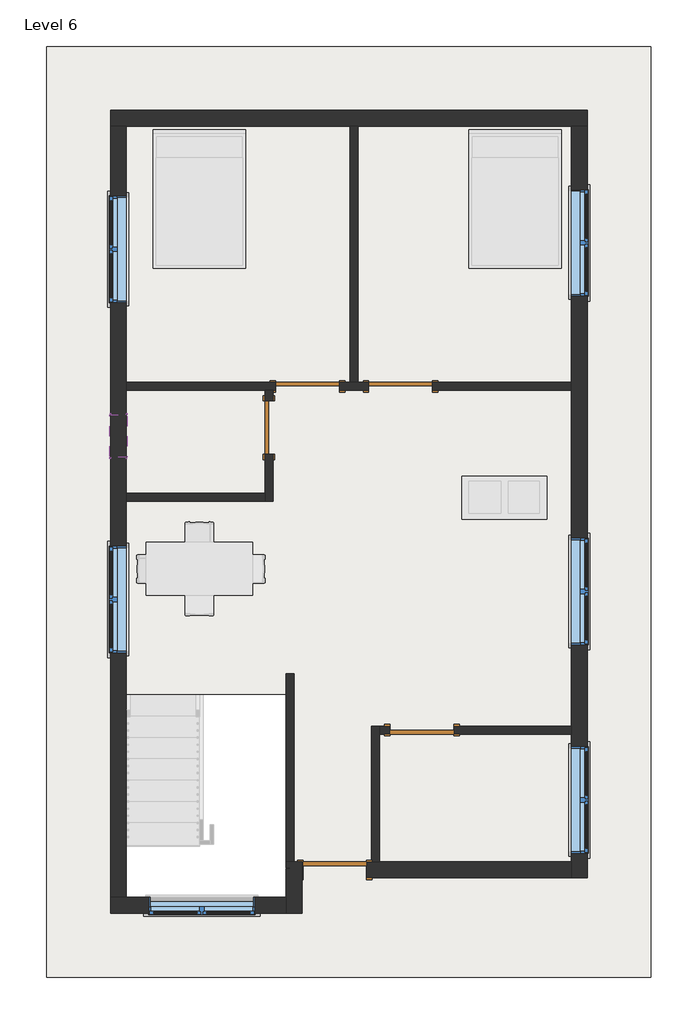
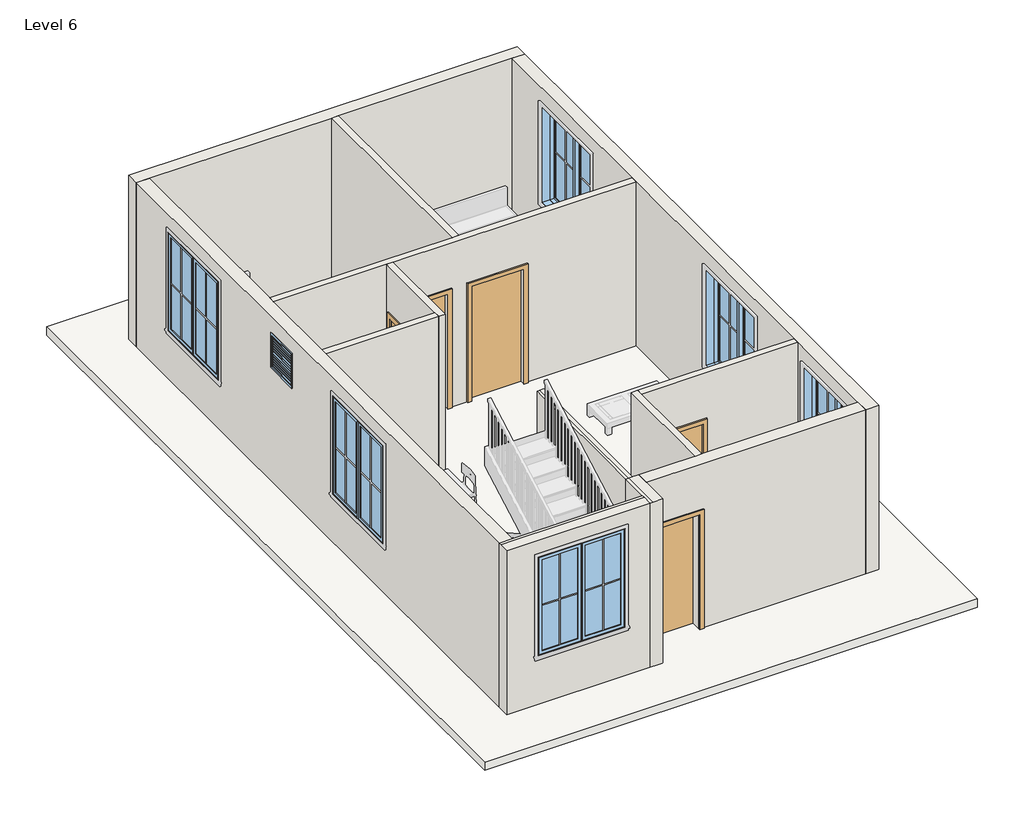
# One storey, part 1 of 3: 13 walls, 7 windows, 5 doors, 1 roof.
"""IFC4 building model written with IfcOpenShell, lengths in millimetres."""

from ifc_helpers import new_model, si_unit, frame, origin, place, context, project, spatial, polyline, outline, extrude, faceted_brep, transform, mapped, element, save
from components import door_214872d5, single_flush_door_3_e5f9f3c4, single_flush_door_3_305aa2a5, single_flush_door_3_0ca8825f, window_casement_double_win_5_f93960c7, window_f2d8fef0

model = new_model("IFC4")

# Units and contexts
model_context = context("Model", 3, world=origin())
ifc_project = project(units=[si_unit("LENGTHUNIT", "METRE", prefix="MILLI")], contexts=[model_context])

# Site, building, storey
site = spatial("IfcSite", under=ifc_project)
building = spatial("IfcBuilding", under=site)
storey = spatial("IfcBuildingStorey", under=building, Name="Level 6", Elevation=15849.6)

# Doors
placement = place(None, origin())
door_shape = door_214872d5(model_context)
element("IfcDoor", 1, ObjectType="Single-Flush : DOOR 2'6\"", at=placement, inside=storey, context=model_context, shape_type="MappedRepresentation", body=[
    mapped(door_shape, transform((-2193.930864, 251.0919982, 15849.6), x_axis=(0.0, 1.0, 0.0), y_axis=(-1.0, 0.0, 0.0), z_axis=(0.0, 0.0, 1.0))),
])
single_flush_door_3_shape = single_flush_door_3_e5f9f3c4(model_context)
element("IfcDoor", 2, ObjectType="Single-Flush : DOOR 3'", at=placement, inside=storey, context=model_context, shape_type="MappedRepresentation", body=[
    mapped(single_flush_door_3_shape, transform((-1641.3962678, 841.6419982, 15849.6), x_axis=(1.0, 0.0, 0.0), y_axis=(0.0, 1.0, 0.0), z_axis=(0.0, 0.0, 1.0))),
])
element("IfcDoor", 3, ObjectType="Single-Flush : DOOR 3'", at=placement, inside=storey, context=model_context, shape_type="MappedRepresentation", body=[
    mapped(single_flush_door_3_shape, transform((-3.180864, -4073.2580018, 15849.6), x_axis=(-1.0, 0.0, 0.0), y_axis=(0.0, -1.0, 0.0), z_axis=(0.0, 0.0, 1.0))),
])
single_flush_door_3_2_shape = single_flush_door_3_305aa2a5(model_context)
element("IfcDoor", 4, ObjectType="Single-Flush : DOOR 3'", at=placement, inside=storey, context=model_context, shape_type="MappedRepresentation", body=[
    mapped(single_flush_door_3_2_shape, transform((-307.980864, 841.6419982, 15849.6), x_axis=(-1.0, 0.0, 0.0), y_axis=(0.0, -1.0, 0.0), z_axis=(0.0, 0.0, 1.0))),
])
single_flush_door_3_3_shape = single_flush_door_3_0ca8825f(model_context)
element("IfcDoor", 5, ObjectType="Single-Flush : DOOR 3'", at=placement, inside=storey, context=model_context, shape_type="MappedRepresentation", body=[
    mapped(single_flush_door_3_3_shape, transform((-1250.955864, -6073.5080018, 15849.6), x_axis=(1.0, 0.0, 0.0), y_axis=(0.0, 1.0, 0.0), z_axis=(0.0, 0.0, 1.0))),
])

# Roof
element("IfcRoof", 6, ObjectType="ROOF 6\"", at=placement, inside=storey, context=model_context, shape_type="SweptSolid", body=[
    extrude(outline(polyline([(3273.419136, 5699.3919982), (3273.419136, -7610.2080018), (-5375.280864, -7610.2080018), (-5375.280864, 5699.3919982), (3273.419136, 5699.3919982)]), holes=[polyline([(-1895.480864, -3571.6080018), (-4232.280864, -3571.6080018), (-4232.280864, -6518.0080018), (-1895.480864, -6518.0080018), (-1895.480864, -3571.6080018)])]), frame((0.0, 0.0, 15697.2), z_axis=(0.0, 0.0, 1.0), x_axis=(1.0, 0.0, 0.0)), (0.0, 0.0, 1.0), 152.4),
])

# Walls
element("IfcWall", 7, ObjectType="WALL 4.5\"", at=placement, inside=storey, context=model_context, shape_type="SweptSolid", body=[
    extrude(outline(polyline([(-1031.880864, 898.7919982), (-1031.880864, 4556.3919982), (-917.580864, 4556.3919982), (-917.580864, 898.7919982), (-1031.880864, 898.7919982)])), frame((0.0, 0.0, 15849.6), z_axis=(0.0, 0.0, 1.0), x_axis=(1.0, 0.0, 0.0)), (0.0, 0.0, 1.0), 3048.0),
])
element("IfcWall", 8, ObjectType="WALL 4.5\"", at=placement, inside=storey, context=model_context, shape_type="Brep", body=[
    faceted_brep([(-765.180864, 898.7919982, 17983.2), (-765.180864, 898.7919982, 15849.6), (-917.580864, 898.7919982, 15849.6), (-1031.880864, 898.7919982, 15849.6), (-1184.1962678, 898.7919982, 15849.6), (-1184.1962678, 898.7919982, 17983.2), (-2098.5962678, 898.7919982, 17983.2), (-2098.5962678, 898.7919982, 15849.6), (-4232.280864, 898.7919982, 15849.6), (-4232.280864, 898.7919982, 18897.6), (-1031.880864, 898.7919982, 18897.6), (-917.580864, 898.7919982, 18897.6), (2130.419136, 898.7919982, 18897.6), (2130.419136, 898.7919982, 15849.6), (149.219136, 898.7919982, 15849.6), (149.219136, 898.7919982, 17983.2), (-1184.1962678, 784.4919982, 15849.6), (-765.180864, 784.4919982, 15849.6), (-765.180864, 784.4919982, 17983.2), (149.219136, 784.4919982, 17983.2), (149.219136, 784.4919982, 15849.6), (2130.419136, 784.4919982, 15849.6), (2130.419136, 784.4919982, 18897.6), (-2136.780864, 784.4919982, 18897.6), (-2251.080864, 784.4919982, 18897.6), (-4232.280864, 784.4919982, 18897.6), (-4232.280864, 784.4919982, 15849.6), (-2251.080864, 784.4919982, 15849.6), (-2136.780864, 784.4919982, 15849.6), (-2098.5962678, 784.4919982, 15849.6), (-2098.5962678, 784.4919982, 17983.2), (-1184.1962678, 784.4919982, 17983.2)], [[[0, 1, 2, 3, 4, 5, 6, 7, 8, 9, 10, 11, 12, 13, 14, 15]], [[16, 17, 18, 19, 20, 21, 22, 23, 24, 25, 26, 27, 28, 29, 30, 31]], [[29, 28, 27, 26, 8, 7]], [[14, 13, 21, 20]], [[4, 3, 2, 1, 17, 16]], [[13, 12, 22, 21]], [[9, 8, 26, 25]], [[5, 4, 16, 31]], [[6, 5, 31, 30]], [[7, 6, 30, 29]], [[18, 17, 1, 0]], [[19, 18, 0, 15]], [[20, 19, 15, 14]], [[12, 11, 10, 9, 25, 24, 23, 22]]]),
])
element("IfcWall", 9, ObjectType="WALL 4.5\"", at=placement, inside=storey, context=model_context, shape_type="Brep", body=[
    faceted_brep([(-2251.080864, 784.4919982, 15849.6), (-2251.080864, 632.0919982, 15849.6), (-2251.080864, 632.0919982, 17983.2), (-2251.080864, -129.9080018, 17983.2), (-2251.080864, -129.9080018, 15849.6), (-2251.080864, -688.7080018, 15849.6), (-2251.080864, -803.0080018, 15849.6), (-2251.080864, -803.0080018, 18897.6), (-2251.080864, -688.7080018, 18897.6), (-2251.080864, 784.4919982, 18897.6), (-2136.780864, 632.0919982, 17983.2), (-2136.780864, 632.0919982, 15849.6), (-2136.780864, 784.4919982, 15849.6), (-2136.780864, 784.4919982, 18897.6), (-2136.780864, -803.0080018, 18897.6), (-2136.780864, -803.0080018, 15849.6), (-2136.780864, -129.9080018, 15849.6), (-2136.780864, -129.9080018, 17983.2)], [[[0, 1, 2, 3, 4, 5, 6, 7, 8, 9]], [[10, 11, 12, 13, 14, 15, 16, 17]], [[16, 15, 6, 5, 4]], [[12, 11, 1, 0]], [[0, 9, 13, 12]], [[7, 6, 15, 14]], [[2, 1, 11, 10]], [[3, 2, 10, 17]], [[4, 3, 17, 16]], [[9, 8, 7, 14, 13]]]),
])
element("IfcWall", 10, ObjectType="WALL 4.5\"", at=placement, inside=storey, context=model_context, shape_type="SweptSolid", body=[
    extrude(outline(polyline([(-4232.280864, -688.7080018), (-2251.080864, -688.7080018), (-2251.080864, -803.0080018), (-4232.280864, -803.0080018), (-4232.280864, -688.7080018)])), frame((0.0, 0.0, 15849.6), z_axis=(0.0, 0.0, 1.0), x_axis=(1.0, 0.0, 0.0)), (0.0, 0.0, 1.0), 3048.0),
])
element("IfcWall", 11, ObjectType="WALL 4.5\"", at=placement, inside=storey, context=model_context, shape_type="Brep", body=[
    faceted_brep([(-1831.980864, -5959.2080018, 15849.6), (-1831.980864, -3266.8080018, 15849.6), (-1831.980864, -3266.8080018, 18897.6), (-1831.980864, -5959.2080018, 18897.6), (-1946.280864, -5959.2080018, 15849.6), (-1946.280864, -5959.2080018, 18897.6), (-1946.280864, -3266.8080018, 18897.6), (-1946.280864, -3266.8080018, 15849.6), (-1895.480864, -3266.8080018, 18897.6), (-1895.480864, -5959.2080018, 18897.6), (-1895.480864, -3571.6080018, 18897.6)], [[[0, 1, 2, 3]], [[4, 5, 6, 7]], [[1, 0, 4, 7]], [[2, 1, 7, 6, 8]], [[0, 3, 9, 5, 4]], [[3, 2, 8, 10, 9]], [[8, 6, 5, 9, 10]]]),
])
element("IfcWall", 12, ObjectType="WALL 4.5\"", at=placement, inside=storey, context=model_context, shape_type="Brep", body=[
    faceted_brep([(-612.780864, -5959.2080018, 15849.6), (-612.780864, -4130.4080018, 15849.6), (-612.780864, -4016.1080018, 15849.6), (-612.780864, -4016.1080018, 18897.6), (-612.780864, -4130.4080018, 18897.6), (-612.780864, -5959.2080018, 18897.6), (-727.080864, -5959.2080018, 15849.6), (-727.080864, -5959.2080018, 18897.6), (-727.080864, -4016.1080018, 18897.6), (-727.080864, -4016.1080018, 15849.6)], [[[0, 1, 2, 3, 4, 5]], [[6, 7, 8, 9]], [[2, 1, 0, 6, 9]], [[0, 5, 7, 6]], [[3, 2, 9, 8]], [[5, 4, 3, 8, 7]]]),
])
element("IfcWall", 13, ObjectType="WALL 4.5\"", at=placement, inside=storey, context=model_context, shape_type="SweptSolid", body=[
    extrude(outline(polyline([(15849.6, -612.780864), (15849.6, -460.380864), (17983.2, -460.380864), (17983.2, 454.019136), (15849.6, 454.019136), (15849.6, 2130.419136), (18897.6, 2130.419136), (18897.6, -612.780864), (15849.6, -612.780864)])), frame((0.0, -4130.4080018, 0.0), z_axis=(0.0, 1.0, 0.0), x_axis=(0.0, 0.0, 1.0)), (0.0, 0.0, 1.0), 114.3),
])
element("IfcWall", 14, ObjectType="WALL 9\"", at=placement, inside=storey, context=model_context, shape_type="Brep", body=[
    faceted_brep([(-4460.880864, 4556.3919982, 15849.6), (-4232.280864, 4556.3919982, 15849.6), (-1031.880864, 4556.3919982, 15849.6), (-917.580864, 4556.3919982, 15849.6), (2130.419136, 4556.3919982, 15849.6), (2359.019136, 4556.3919982, 15849.6), (2359.019136, 4556.3919982, 18897.6), (2130.419136, 4556.3919982, 18897.6), (-917.580864, 4556.3919982, 18897.6), (-1031.880864, 4556.3919982, 18897.6), (-4232.280864, 4556.3919982, 18897.6), (-4460.880864, 4556.3919982, 18897.6), (-4460.880864, 4784.9919982, 15849.6), (-4460.880864, 4784.9919982, 18897.6), (2359.019136, 4784.9919982, 18897.6), (2359.019136, 4784.9919982, 15849.6)], [[[0, 1, 2, 3, 4, 5, 6, 7, 8, 9, 10, 11]], [[12, 13, 14, 15]], [[5, 4, 3, 2, 1, 0, 12, 15]], [[6, 5, 15, 14]], [[0, 11, 13, 12]], [[11, 10, 9, 8, 7, 6, 14, 13]]]),
])
element("IfcWall", 15, ObjectType="WALL 9\"", at=placement, inside=storey, context=model_context, shape_type="Brep", body=[
    faceted_brep([(2130.419136, 4556.3919982, 15849.6), (2130.419136, 898.7919982, 15849.6), (2130.419136, 784.4919982, 15849.6), (2130.419136, -4016.1080018, 15849.6), (2130.419136, -4130.4080018, 15849.6), (2130.419136, -5959.2080018, 15849.6), (2130.419136, -6187.8080018, 15849.6), (2130.419136, -6187.8080018, 18897.6), (2130.419136, -5959.2080018, 18897.6), (2130.419136, -4130.4080018, 18897.6), (2130.419136, -4016.1080018, 18897.6), (2130.419136, 784.4919982, 18897.6), (2130.419136, 898.7919982, 18897.6), (2130.419136, 4556.3919982, 18897.6), (2130.419136, -5835.3830018, 18592.8), (2130.419136, -5835.3830018, 16764.0), (2130.419136, -4311.3830018, 16764.0), (2130.419136, -4311.3830018, 18592.8), (2130.419136, -2854.0580018, 18592.8), (2130.419136, -2854.0580018, 16764.0), (2130.419136, -1330.0580018, 16764.0), (2130.419136, -1330.0580018, 18592.8), (2130.419136, 2130.6919982, 18592.8), (2130.419136, 2130.6919982, 16764.0), (2130.419136, 3654.6919982, 16764.0), (2130.419136, 3654.6919982, 18592.8), (2359.019136, 4556.3919982, 15849.6), (2359.019136, 4556.3919982, 18897.6), (2359.019136, -6187.8080018, 18897.6), (2359.019136, -6187.8080018, 15849.6), (2359.019136, -5835.3830018, 18592.8), (2359.019136, -4311.3830018, 18592.8), (2359.019136, -4311.3830018, 16764.0), (2359.019136, -5835.3830018, 16764.0), (2359.019136, -2854.0580018, 18592.8), (2359.019136, -1330.0580018, 18592.8), (2359.019136, -1330.0580018, 16764.0), (2359.019136, -2854.0580018, 16764.0), (2359.019136, 2130.6919982, 18592.8), (2359.019136, 3654.6919982, 18592.8), (2359.019136, 3654.6919982, 16764.0), (2359.019136, 2130.6919982, 16764.0)], [[[0, 1, 2, 3, 4, 5, 6, 7, 8, 9, 10, 11, 12, 13], [14, 15, 16, 17], [18, 19, 20, 21], [22, 23, 24, 25]], [[26, 27, 28, 29], [30, 31, 32, 33], [34, 35, 36, 37], [38, 39, 40, 41]], [[6, 5, 4, 3, 2, 1, 0, 26, 29]], [[0, 13, 27, 26]], [[7, 6, 29, 28]], [[15, 14, 30, 33]], [[16, 15, 33, 32]], [[17, 16, 32, 31]], [[14, 17, 31, 30]], [[19, 18, 34, 37]], [[20, 19, 37, 36]], [[21, 20, 36, 35]], [[18, 21, 35, 34]], [[23, 22, 38, 41]], [[24, 23, 41, 40]], [[25, 24, 40, 39]], [[22, 25, 39, 38]], [[13, 12, 11, 10, 9, 8, 7, 28, 27]]]),
])
element("IfcWall", 16, ObjectType="WALL 9\"", at=placement, inside=storey, context=model_context, shape_type="Brep", body=[
    faceted_brep([(2130.419136, -5959.2080018, 15849.6), (-612.780864, -5959.2080018, 15849.6), (-727.080864, -5959.2080018, 15849.6), (-793.755864, -5959.2080018, 15849.6), (-793.755864, -5959.2080018, 17983.2), (-1708.155864, -5959.2080018, 17983.2), (-1708.155864, -5959.2080018, 15849.6), (-1717.680864, -5959.2080018, 15849.6), (-1717.680864, -5959.2080018, 18897.6), (-727.080864, -5959.2080018, 18897.6), (-612.780864, -5959.2080018, 18897.6), (2130.419136, -5959.2080018, 18897.6), (-793.755864, -6187.8080018, 17983.2), (-793.755864, -6187.8080018, 15849.6), (2130.419136, -6187.8080018, 15849.6), (2130.419136, -6187.8080018, 18897.6), (-1717.680864, -6187.8080018, 18897.6), (-1717.680864, -6187.8080018, 15849.6), (-1708.155864, -6187.8080018, 15849.6), (-1708.155864, -6187.8080018, 17983.2)], [[[0, 1, 2, 3, 4, 5, 6, 7, 8, 9, 10, 11]], [[12, 13, 14, 15, 16, 17, 18, 19]], [[18, 17, 7, 6]], [[14, 13, 3, 2, 1, 0]], [[0, 11, 15, 14]], [[8, 7, 17, 16]], [[4, 3, 13, 12]], [[5, 4, 12, 19]], [[6, 5, 19, 18]], [[11, 10, 9, 8, 16, 15]]]),
])
element("IfcWall", 17, ObjectType="WALL 9\"", at=placement, inside=storey, context=model_context, shape_type="Brep", body=[
    faceted_brep([(-1946.280864, -5959.2080018, 15849.6), (-1946.280864, -6467.2080018, 15849.6), (-1946.280864, -6695.8080018, 15849.6), (-1946.280864, -6695.8080018, 18897.6), (-1946.280864, -6467.2080018, 18897.6), (-1946.280864, -5959.2080018, 18897.6), (-1717.680864, -5959.2080018, 15849.6), (-1717.680864, -5959.2080018, 18897.6), (-1717.680864, -6187.8080018, 18897.6), (-1717.680864, -6695.8080018, 18897.6), (-1717.680864, -6695.8080018, 15849.6), (-1717.680864, -6187.8080018, 15849.6), (-1831.980864, -5959.2080018, 15849.6), (-1895.480864, -5959.2080018, 18897.6), (-1831.980864, -5959.2080018, 18897.6), (-1895.480864, -6695.8080018, 18897.6), (-1895.480864, -6518.0080018, 18897.6)], [[[0, 1, 2, 3, 4, 5]], [[6, 7, 8, 9, 10, 11]], [[2, 1, 0, 12, 6, 11, 10]], [[0, 5, 13, 14, 7, 6, 12]], [[3, 2, 10, 9, 15]], [[5, 4, 3, 15, 16, 13]], [[15, 9, 8, 7, 14, 13, 16]]]),
])
element("IfcWall", 18, ObjectType="WALL 9\"", at=placement, inside=storey, context=model_context, shape_type="Brep", body=[
    faceted_brep([(-1946.280864, -6467.2080018, 15849.6), (-4232.280864, -6467.2080018, 15849.6), (-4460.880864, -6467.2080018, 15849.6), (-4460.880864, -6467.2080018, 18897.6), (-4232.280864, -6467.2080018, 18897.6), (-1946.280864, -6467.2080018, 18897.6), (-3914.780864, -6467.2080018, 18592.8), (-3914.780864, -6467.2080018, 16764.0), (-2390.780864, -6467.2080018, 16764.0), (-2390.780864, -6467.2080018, 18592.8), (-1946.280864, -6695.8080018, 15849.6), (-1946.280864, -6695.8080018, 18897.6), (-4460.880864, -6695.8080018, 18897.6), (-4460.880864, -6695.8080018, 15849.6), (-3914.780864, -6695.8080018, 18592.8), (-2390.780864, -6695.8080018, 18592.8), (-2390.780864, -6695.8080018, 16764.0), (-3914.780864, -6695.8080018, 16764.0), (-1946.280864, -6518.0080018, 18897.6), (-4460.880864, -6518.0080018, 18897.6), (-4232.280864, -6518.0080018, 18897.6)], [[[0, 1, 2, 3, 4, 5], [6, 7, 8, 9]], [[10, 11, 12, 13], [14, 15, 16, 17]], [[2, 1, 0, 10, 13]], [[0, 5, 18, 11, 10]], [[3, 2, 13, 12, 19]], [[7, 6, 14, 17]], [[8, 7, 17, 16]], [[9, 8, 16, 15]], [[6, 9, 15, 14]], [[5, 4, 3, 19, 20, 18]], [[19, 12, 11, 18, 20]]]),
])
element("IfcWall", 19, ObjectType="WALL 9\"", at=placement, inside=storey, context=model_context, shape_type="Brep", body=[
    faceted_brep([(-4232.280864, -6467.2080018, 15849.6), (-4232.280864, -803.0080018, 15849.6), (-4232.280864, -688.7080018, 15849.6), (-4232.280864, 784.4919982, 15849.6), (-4232.280864, 898.7919982, 15849.6), (-4232.280864, 4556.3919982, 15849.6), (-4232.280864, 4556.3919982, 18897.6), (-4232.280864, 898.7919982, 18897.6), (-4232.280864, 784.4919982, 18897.6), (-4232.280864, -688.7080018, 18897.6), (-4232.280864, -803.0080018, 18897.6), (-4232.280864, -3571.6080018, 18897.6), (-4232.280864, -6467.2080018, 18897.6), (-4232.280864, -1445.1400081, 18592.8), (-4232.280864, -1445.1400081, 16764.0), (-4232.280864, -2969.1400081, 16764.0), (-4232.280864, -2969.1400081, 18592.8), (-4232.280864, 3562.6287133, 18592.8), (-4232.280864, 3562.6287133, 16764.0), (-4232.280864, 2038.6287133, 16764.0), (-4232.280864, 2038.6287133, 18592.8), (-4232.280864, -174.3580018, 18592.8), (-4232.280864, 435.2419982, 18592.8), (-4232.280864, 435.2419982, 17983.2), (-4232.280864, -174.3580018, 17983.2), (-4460.880864, -6467.2080018, 15849.6), (-4460.880864, -6467.2080018, 18897.6), (-4460.880864, 4556.3919982, 18897.6), (-4460.880864, 4556.3919982, 15849.6), (-4460.880864, -1445.1400081, 18592.8), (-4460.880864, -2969.1400081, 18592.8), (-4460.880864, -2969.1400081, 16764.0), (-4460.880864, -1445.1400081, 16764.0), (-4460.880864, 3562.6287133, 18592.8), (-4460.880864, 2038.6287133, 18592.8), (-4460.880864, 2038.6287133, 16764.0), (-4460.880864, 3562.6287133, 16764.0), (-4460.880864, -174.3580018, 18592.8), (-4460.880864, -174.3580018, 17983.2), (-4460.880864, 435.2419982, 17983.2), (-4460.880864, 435.2419982, 18592.8)], [[[0, 1, 2, 3, 4, 5, 6, 7, 8, 9, 10, 11, 12], [13, 14, 15, 16], [17, 18, 19, 20], [21, 22, 23, 24]], [[25, 26, 27, 28], [29, 30, 31, 32], [33, 34, 35, 36], [37, 38, 39, 40]], [[5, 4, 3, 2, 1, 0, 25, 28]], [[6, 5, 28, 27]], [[0, 12, 26, 25]], [[14, 13, 29, 32]], [[15, 14, 32, 31]], [[16, 15, 31, 30]], [[13, 16, 30, 29]], [[18, 17, 33, 36]], [[19, 18, 36, 35]], [[20, 19, 35, 34]], [[17, 20, 34, 33]], [[38, 37, 21, 24]], [[39, 38, 24, 23]], [[40, 39, 23, 22]], [[37, 40, 22, 21]], [[12, 11, 10, 9, 8, 7, 6, 27, 26]]]),
])

# Windows
window_casement_double_win_5_shape = window_casement_double_win_5_f93960c7(model_context)
element("IfcWindow", 20, ObjectType="Window-Casement-Double : WIN 5'", at=placement, inside=storey, context=model_context, shape_type="MappedRepresentation", body=[
    mapped(window_casement_double_win_5_shape, transform((-3152.780864, -6581.5080018, 15849.6), x_axis=(-1.0, 0.0, 0.0), y_axis=(0.0, -1.0, 0.0), z_axis=(0.0, 0.0, 1.0))),
])
element("IfcWindow", 21, ObjectType="Window-Casement-Double : WIN 5'", at=placement, inside=storey, context=model_context, shape_type="MappedRepresentation", body=[
    mapped(window_casement_double_win_5_shape, transform((2244.719136, -5073.3830018, 15849.6), x_axis=(0.0, -1.0, 0.0), y_axis=(1.0, 0.0, 0.0), z_axis=(0.0, 0.0, 1.0))),
])
element("IfcWindow", 22, ObjectType="Window-Casement-Double : WIN 5'", at=placement, inside=storey, context=model_context, shape_type="MappedRepresentation", body=[
    mapped(window_casement_double_win_5_shape, transform((2244.719136, -2092.0580018, 15849.6), x_axis=(0.0, -1.0, 0.0), y_axis=(1.0, 0.0, 0.0), z_axis=(0.0, 0.0, 1.0))),
])
element("IfcWindow", 23, ObjectType="Window-Casement-Double : WIN 5'", at=placement, inside=storey, context=model_context, shape_type="MappedRepresentation", body=[
    mapped(window_casement_double_win_5_shape, transform((-4346.580864, -2207.1400081, 15849.6), x_axis=(0.0, 1.0, 0.0), y_axis=(-1.0, 0.0, 0.0), z_axis=(0.0, 0.0, 1.0))),
])
element("IfcWindow", 24, ObjectType="Window-Casement-Double : WIN 5'", at=placement, inside=storey, context=model_context, shape_type="MappedRepresentation", body=[
    mapped(window_casement_double_win_5_shape, transform((2244.719136, 2892.6919982, 15849.6), x_axis=(0.0, -1.0, 0.0), y_axis=(1.0, 0.0, 0.0), z_axis=(0.0, 0.0, 1.0))),
])
element("IfcWindow", 25, ObjectType="Window-Casement-Double : WIN 5'", at=placement, inside=storey, context=model_context, shape_type="MappedRepresentation", body=[
    mapped(window_casement_double_win_5_shape, transform((-4346.580864, 2800.6287133, 15849.6), x_axis=(0.0, 1.0, 0.0), y_axis=(-1.0, 0.0, 0.0), z_axis=(0.0, 0.0, 1.0))),
])
window_shape = window_f2d8fef0(model_context)
element("IfcWindow", 26, ObjectType="Window-Louvers : 24\" x 24\"", at=placement, inside=storey, context=model_context, shape_type="MappedRepresentation", body=[
    mapped(window_shape, transform((-4352.930864, 130.4419982, 17068.8), x_axis=(0.0, 1.0, 0.0), y_axis=(-1.0, 0.0, 0.0), z_axis=(0.0, 0.0, 1.0))),
])

save(model, "model.ifc")

# Revit data of these elements
# Type "Single-Flush : DOOR 2'6\""
#   Type Mark = "9"
#   Construction Type Id = "MDOOR"
#   Assembly Code = "C1020"
#   Analytic Construction = "Metal"
#   Thickness = 0' - 2"
#   Heat Transfer Coefficient (U) = 0.651978 BTU/(h·ft²·°F)
#   Height = 7' - 0"
#   Trim Projection Ext = 0' - 1"
#   Trim Projection Int = 0' - 1"
#   Trim Width = 0' - 3"
#   Width = 2' - 6"
#   Define Thermal Properties by = 1
#   Door Material = Door - Panel
#   Frame Material = Door - Frame
#   Visual Light Transmittance = 0
#   Solar Heat Gain Coefficient = 0
#   Function = (empty or 0)
#   Wall Closure = (empty or 0)
# Type "Single-Flush : DOOR 3'"
#   Type Mark = "8"
#   Construction Type Id = "MDOOR"
#   Assembly Code = "C1020"
#   Analytic Construction = "Metal"
#   Thickness = 0' - 2"
#   Heat Transfer Coefficient (U) = 0.651978 BTU/(h·ft²·°F)
#   Height = 7' - 0"
#   Trim Projection Ext = 0' - 1"
#   Trim Projection Int = 0' - 1"
#   Trim Width = 0' - 3"
#   Width = 3' - 0"
#   Define Thermal Properties by = 1
#   Door Material = Door - Panel
#   Frame Material = Door - Frame
#   Visual Light Transmittance = 0
#   Solar Heat Gain Coefficient = 0
#   Function = (empty or 0)
#   Wall Closure = (empty or 0)
# Type "ROOF 6\""
#   Assembly Code = "B1020"
#   Layers, outside or top first: 0' - 6" no material (function 1)
# Type "WALL 4.5\""
#   Assembly Code = "B2010"
#   Layers, outside or top first: 0' - 4 1/2" no material (function 1)
# Type "WALL 9\""
#   Assembly Code = "B2010"
#   Layers, outside or top first: 0' - 9" no material (function 1)
# Type "Window-Casement-Double : WIN 5'"
#   Type Mark = "18"
#   Fire Rating = "0.5h"
#   Assembly Code = "B2020100"
#   Analytic Construction = "Double glazing - domestic"
#   Frame Extension [instance default] = 0' - 0 1/4"
#   Window Inset [instance default] = 0' - 0"
#   Wall Thickness [instance default] = 0' - 6"
#   Interior Wall Closure [instance default] = 0' - 2 1/4"
#   Half Width = 2' - 6"
#   Visual Light Transmittance = 0.81
#   Thermal Resistance (R) = 1.8146 (h·ft²·°F)/BTU
#   Solar Heat Gain Coefficient = 0.76
#   Rough Width = 5' - 0 1/2"
#   Rough Height = 6' - 0 1/2"
#   Height = 6' - 0"
#   Heat Transfer Coefficient (U) = 0.5511 BTU/(h·ft²·°F)
#   Exterior Wall Closure [instance default] = 0' - 1 1/4"
#   Extension Jamb [instance default] = 0' - 2 1/4"
#   Default Sill Height = 3' - 0"
#   Width = 5' - 0"
#   Muntin Visibility = yes
#   Interior Trim Visibility [instance default] = yes
#   Exterior Trim Visibility [instance default] = yes
#   Extension Jamb Visibility [instance default] = yes
#   Interior Trim Material = Wood - Stained
#   Muntin Pattern = Muntin Pattern_2x2 : Muntin Pattern_2x2
#   Interior Trim = Trim-Window-Interior-Flat : Picture Frame
#   Interior Frame Material = Wood - Stained
#   Glass Panel Material = Glass
#   Exterior Trim Material = Clad - White
#   Exterior Trim = Trim-Window-Exterior-Flat : with Sill
#   Exterior Frame Material = Clad - White
#   Wall Closure = (empty or 0)
# Type "Window-Louvers : 24\" x 24\""
#   Type Mark = "19"
#   Construction Type Id = "GSP4R"
#   Assembly Code = "B20"
#   Analytic Construction = "1/8 in Pilkington single glazing"
#   Visual Light Transmittance = 0.9
#   Thermal Resistance (R) = 1.53941 (h·ft²·°F)/BTU
#   Solar Heat Gain Coefficient = 0.78
#   Max Height = 1' - 11.74264"
#   Height = 2' - 0"
#   Heat Transfer Coefficient (U) = 0.6496 BTU/(h·ft²·°F)
#   Blade Width [instance default] = 1' - 10 1/2"
#   Blade Vertical Thickness = 0' - 0.35355"
#   Blade Thickness = 0' - 0 1/4"
#   Blade Spacing = 0' - 1 1/2"
#   Blade Height = 0' - 1.85355"
#   Blade Depth = 0' - 3"
#   Blade Angle = 45.00°
#   Default Sill Height = 3' - 0"
#   Trim Projection_Exterior = 0' - 0 1/2"
#   Trim Projection_Interior = 0' - 0 1/2"
#   Trim Width_Exterior = 0' - 1 1/2"
#   Trim Width_Interior = 0' - 1 1/2"
#   Width = 2' - 0"
#   Max Blade Count = 12
#   Define Thermal Properties by = 1
#   Blade Count = 12
#   Frame Material = Birch
#   Louver Material = Birch
#   Trim Exterior Material = Birch
#   Trim Interior Material = Birch
#   Wall Closure = (empty or 0)
# Element 1 (IfcDoor, "Single-Flush : DOOR 2'6\"")
#   Phase Created = New Construction
#   Materials on its faces: "Door - Frame", "Door - Panel"
# Elements 2, 3, 4, 5 (IfcDoor, "Single-Flush : DOOR 3'")
#   Phase Created = New Construction
#   Materials on its faces: "Door - Frame", "Door - Panel"
# Element 6 (IfcRoof, "ROOF 6\"")
#   built-in parameter 1001705 = 52 (stored number, unit not read)
#   built-in parameter 1001701 = -0.5 (stored number, unit not read)
#   built-in parameter 1001710 = 33615
#   Phase Created = New Construction
#   Materials on its faces: "Copper", "Wood - Stained"
# Elements 7, 8, 9, 10, 12, 13 (IfcWall, "WALL 4.5\"")
#   Top Offset = 0' - 0"
#   Base Offset = 0' - 0"
#   Unconnected Height = 10' - 0"
#   wall height = 10' - 0"
#   Phase Created = New Construction
#   Base Constraint = Level 6
#   Materials on its faces: "Default Wall"
# Element 11 (IfcWall, "WALL 4.5\"")
#   Top Offset = 0' - 0"
#   Base Offset = 0' - 0"
#   Unconnected Height = 10' - 0"
#   wall height = 10' - 0"
#   Phase Created = New Construction
#   Base Constraint = Level 6
#   Materials on its faces: "Default Wall", "Copper"
# Elements 14, 15, 16 (IfcWall, "WALL 9\"")
#   Top Offset = 0' - 0"
#   Base Offset = 0' - 0"
#   Unconnected Height = 10' - 0"
#   wall height = 10' - 0"
#   Phase Created = New Construction
#   Base Constraint = Level 6
#   Materials on its faces: "Default Wall"
# Elements 17, 18, 19 (IfcWall, "WALL 9\"")
#   Top Offset = 0' - 0"
#   Base Offset = 0' - 0"
#   Unconnected Height = 10' - 0"
#   wall height = 10' - 0"
#   Phase Created = New Construction
#   Base Constraint = Level 6
#   Materials on its faces: "Default Wall", "Copper"
# Element 20 (IfcWindow, "Window-Casement-Double : WIN 5'")
#   Mark = "36"
#   Window Inset = 0' - 0"
#   Interior Wall Closure = 0' - 2 1/4"
#   Frame Extension = 0' - 0 1/4"
#   Exterior Wall Closure = 0' - 1 1/4"
#   Interior Trim Visibility = yes
#   Exterior Trim Visibility = yes
#   Phase Created = New Construction
#   Materials on its faces: "Wood - Stained", "Glass", "Clad - White"
# Element 21 (IfcWindow, "Window-Casement-Double : WIN 5'")
#   Mark = "37"
#   Window Inset = 0' - 0"
#   Interior Wall Closure = 0' - 2 1/4"
#   Frame Extension = 0' - 0 1/4"
#   Exterior Wall Closure = 0' - 1 1/4"
#   Interior Trim Visibility = yes
#   Exterior Trim Visibility = yes
#   Phase Created = New Construction
#   Materials on its faces: "Wood - Stained", "Glass", "Clad - White"
# Element 22 (IfcWindow, "Window-Casement-Double : WIN 5'")
#   Mark = "38"
#   Window Inset = 0' - 0"
#   Interior Wall Closure = 0' - 2 1/4"
#   Frame Extension = 0' - 0 1/4"
#   Exterior Wall Closure = 0' - 1 1/4"
#   Interior Trim Visibility = yes
#   Exterior Trim Visibility = yes
#   Phase Created = New Construction
#   Materials on its faces: "Wood - Stained", "Glass", "Clad - White"
# Element 23 (IfcWindow, "Window-Casement-Double : WIN 5'")
#   Mark = "39"
#   Window Inset = 0' - 0"
#   Interior Wall Closure = 0' - 2 1/4"
#   Frame Extension = 0' - 0 1/4"
#   Exterior Wall Closure = 0' - 1 1/4"
#   Interior Trim Visibility = yes
#   Exterior Trim Visibility = yes
#   Phase Created = New Construction
#   Materials on its faces: "Wood - Stained", "Glass", "Clad - White"
# Element 24 (IfcWindow, "Window-Casement-Double : WIN 5'")
#   Mark = "40"
#   Window Inset = 0' - 0"
#   Interior Wall Closure = 0' - 2 1/4"
#   Frame Extension = 0' - 0 1/4"
#   Exterior Wall Closure = 0' - 1 1/4"
#   Interior Trim Visibility = yes
#   Exterior Trim Visibility = yes
#   Phase Created = New Construction
#   Materials on its faces: "Wood - Stained", "Glass", "Clad - White"
# Element 25 (IfcWindow, "Window-Casement-Double : WIN 5'")
#   Mark = "41"
#   Window Inset = 0' - 0"
#   Interior Wall Closure = 0' - 2 1/4"
#   Frame Extension = 0' - 0 1/4"
#   Exterior Wall Closure = 0' - 1 1/4"
#   Interior Trim Visibility = yes
#   Exterior Trim Visibility = yes
#   Phase Created = New Construction
#   Materials on its faces: "Wood - Stained", "Glass", "Clad - White"
# Element 26 (IfcWindow, "Window-Louvers : 24\" x 24\"")
#   Mark = "42"
#   Blade Width = 1' - 10 1/2"
#   Phase Created = New Construction
#   Materials on its faces: "Birch"
# Materials
#   "Door - Panel": class "Wood", colour RGB 210 159 95, transparency 0, Cost = 0
#   "Door - Frame": colour RGB 118 70 51, transparency 0, Cost = 0
#   "Wood - Stained": class "Wood", colour RGB 224 178 126, transparency 0, Cost = 0
#   "Glass": class "Glass", colour RGB 0 128 192, transparency 0.75, Description = "Soda Lime Glass", Cost = 0
#   "Clad - White": class "Wood", colour RGB 242 242 238, transparency 0, Cost = 0
#   "Birch": class "Wood", colour RGB 224 178 126, transparency 0, Description = "Betula Alleghaniensis", Cost = 0
#   "Copper": class "Metal", colour RGB 0 0 0, transparency 0, Description = "Copper, matte finish", Cost = 0
#   "Default Wall": colour RGB 128 128 128, transparency 0, Cost = 0
